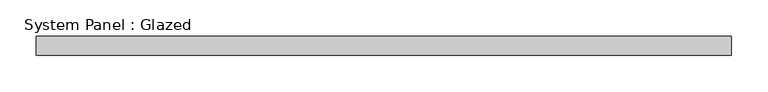
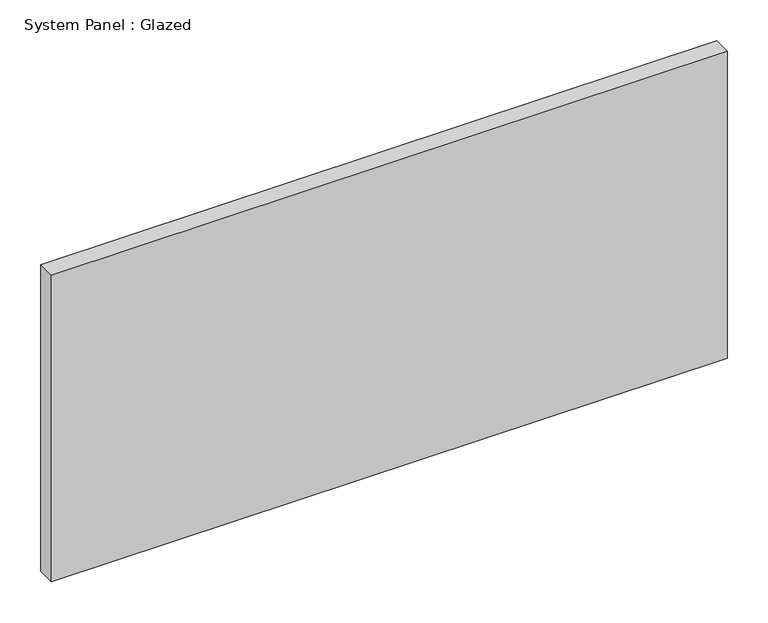
"""IFC4 building model written with IfcOpenShell, lengths in millimetres: plate geometry, System Panel : Glazed."""

from ifc_helpers import new_model, si_unit, origin, origin_with_axes, place, context, project, spatial, polyline, outline, extrude, source, transform, mapped, element, save


def system_panel_glazed_cc3a876e(model_context):
    return source(origin(), model_context, "Body", "SweptSolid", [
        extrude(outline(polyline([(476.25, -44.45), (-476.25, -44.45), (-476.25, -19.05), (476.25, -19.05), (476.25, -44.45)])), origin_with_axes(), (0.0, 0.0, 1.0), 457.2),
    ])


if __name__ == "__main__":
    model = new_model("IFC4")
    model_context = context("Model", 3, world=origin())
    ifc_project = project(units=[si_unit("LENGTHUNIT", "METRE", prefix="MILLI")], contexts=[model_context])
    site = spatial("IfcSite", under=ifc_project)
    building = spatial("IfcBuilding", under=site)
    placement = place(None, origin())
    system_panel_glazed_shape = system_panel_glazed_cc3a876e(model_context)
    element("IfcPlate", 1, ObjectType="System Panel : Glazed", at=placement, inside=building, context=model_context, shape_type="MappedRepresentation", body=[
        mapped(system_panel_glazed_shape, transform((0.0, 0.0, 0.0), x_axis=(1.0, 0.0, 0.0), y_axis=(0.0, 1.0, 0.0), z_axis=(0.0, 0.0, 1.0))),
    ])
    save(model, "model.ifc")

# Revit data of these elements
# Type "System Panel : Glazed"
#   Construction Type Id = "GSP4R"
#   Analytic Construction = "1/8 in Pilkington single glazing"
#   Visual Light Transmittance = 0.9
#   Solar Heat Gain Coefficient = 0.86
#   Heat Transfer Coefficient (U) = 1.18115 BTU/(h·ft²·°F)
#   Define Thermal Properties by = 1
# Element 1 (IfcPlate, "System Panel : Glazed")
#   Materials on its faces: "Glass"
# Materials
#   "Glass": class "Glass", colour RGB 0 128 192, transparency 0.75, Description = "Soda Lime Glass", Cost = 0
